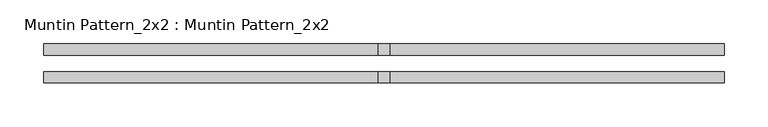
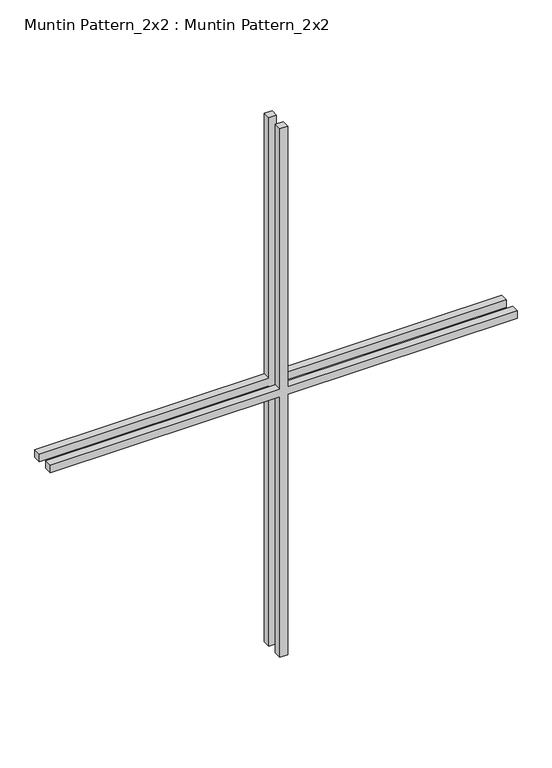
"""IFC4 building model written with IfcOpenShell, lengths in millimetres: proxy geometry, Muntin Pattern_2x2 : Muntin Pattern_2x2."""

from ifc_helpers import new_model, si_unit, frame, origin, place, context, project, spatial, polyline, outline, extrude, source, transform, mapped, element, save


def muntin_pattern_2x2_muntin_pattern_2x2_3e21365d(model_context):
    return source(origin(), model_context, "Body", "SweptSolid", [
        extrude(outline(polyline([(469.9, -6.35), (469.9, -387.35), (457.2, -387.35), (457.2, -6.35), (0.0, -6.35), (0.0, 6.35), (457.2, 6.35), (457.2, 387.35), (469.9, 387.35), (469.9, 6.35), (927.1, 6.35), (927.1, -6.35), (469.9, -6.35)])), frame((0.0, 9.525, 0.0), z_axis=(0.0, 1.0, 0.0), x_axis=(0.0, 0.0, 1.0)), (0.0, 0.0, 1.0), 12.7),
        extrude(outline(polyline([(469.9, -6.35), (469.9, -387.35), (457.2, -387.35), (457.2, -6.35), (0.0, -6.35), (0.0, 6.35), (457.2, 6.35), (457.2, 387.35), (469.9, 387.35), (469.9, 6.35), (927.1, 6.35), (927.1, -6.35), (469.9, -6.35)])), frame((0.0, -22.225, 0.0), z_axis=(0.0, 1.0, 0.0), x_axis=(0.0, 0.0, 1.0)), (0.0, 0.0, 1.0), 12.7),
    ])


if __name__ == "__main__":
    model = new_model("IFC4")
    model_context = context("Model", 3, world=origin())
    ifc_project = project(units=[si_unit("LENGTHUNIT", "METRE", prefix="MILLI")], contexts=[model_context])
    site = spatial("IfcSite", under=ifc_project)
    building = spatial("IfcBuilding", under=site)
    placement = place(None, origin())
    muntin_pattern_2x2_muntin_pattern_2x2_shape = muntin_pattern_2x2_muntin_pattern_2x2_3e21365d(model_context)
    element("IfcBuildingElementProxy", 1, Name="Muntin Pattern_2x2 : Muntin Pattern_2x2", ObjectType="Muntin Pattern_2x2 : Muntin Pattern_2x2", at=placement, inside=building, context=model_context, shape_type="MappedRepresentation", body=[
        mapped(muntin_pattern_2x2_muntin_pattern_2x2_shape, transform((0.0, 0.0, 0.0), x_axis=(1.0, 0.0, 0.0), y_axis=(0.0, 1.0, 0.0), z_axis=(0.0, 0.0, 1.0))),
    ])
    save(model, "model.ifc")

# Revit data of these elements
# Type "Muntin Pattern_2x2 : Muntin Pattern_2x2"
#   Width [instance default] = 4' - 0"
#   Thickness = 0' - 0 1/2"
#   Height [instance default] = 4' - 0"
#   Distance = 0' - 0 3/4"
#   Interior Material [instance default] = none
#   Exterior Material [instance default] = none
#   Default Elevation = 0
# Element 1 (IfcBuildingElementProxy, "Muntin Pattern_2x2 : Muntin Pattern_2x2")
#   Width = 2' - 6 1/2"
#   Height = 3' - 0 1/2"
#   Interior Material = Wood - Stained
#   Exterior Material = Clad - White
#   Materials on its faces: "Clad - White", "Wood - Stained"
# Materials
#   "Clad - White": class "Wood", colour RGB 242 242 238, transparency 0, Cost = 0
#   "Wood - Stained": class "Wood", colour RGB 224 178 126, transparency 0, Cost = 0
